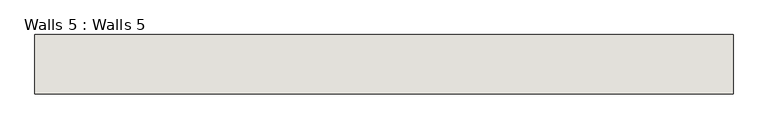
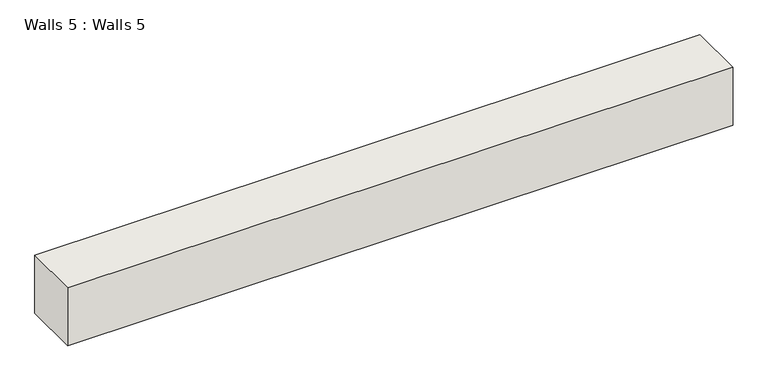
"""IFC4 building model written with IfcOpenShell, lengths in millimetres: wall geometry, Walls 5 : Walls 5."""

from ifc_helpers import new_model, si_unit, frame, origin, place, context, project, spatial, polyline, outline, extrude, source, transform, mapped, element, save


def walls_5_walls_5_63f74a62(model_context):
    return source(origin(), model_context, "Body", "SweptSolid", [
        extrude(outline(polyline([(1448.5864069, -3773.1803698), (-2702.0878119, -3773.1803698), (-2702.0878119, -3420.8536983), (1448.5864069, -3420.8536983), (1448.5864069, -3773.1803698)])), frame((0.0, 0.0, 3048.0), z_axis=(0.0, 0.0, 1.0), x_axis=(1.0, 0.0, 0.0)), (0.0, 0.0, 1.0), 383.083015),
    ])


if __name__ == "__main__":
    model = new_model("IFC4")
    model_context = context("Model", 3, world=origin())
    ifc_project = project(units=[si_unit("LENGTHUNIT", "METRE", prefix="MILLI")], contexts=[model_context])
    site = spatial("IfcSite", under=ifc_project)
    building = spatial("IfcBuilding", under=site)
    placement = place(None, origin())
    walls_5_walls_5_shape = walls_5_walls_5_63f74a62(model_context)
    element("IfcWall", 1, ObjectType="Walls 5 : Walls 5", at=placement, inside=building, context=model_context, shape_type="MappedRepresentation", body=[
        mapped(walls_5_walls_5_shape, transform((0.0, 0.0, 0.0), x_axis=(1.0, 0.0, 0.0), y_axis=(0.0, 1.0, 0.0), z_axis=(0.0, 0.0, 1.0))),
    ])
    save(model, "model.ifc")

# Revit data of these elements
# Element 1 (IfcWall, "Walls 5 : Walls 5")
#   Materials on its faces: "Default Wall"
# Materials
#   "Default Wall": colour RGB 80 80 80, transparency 0
